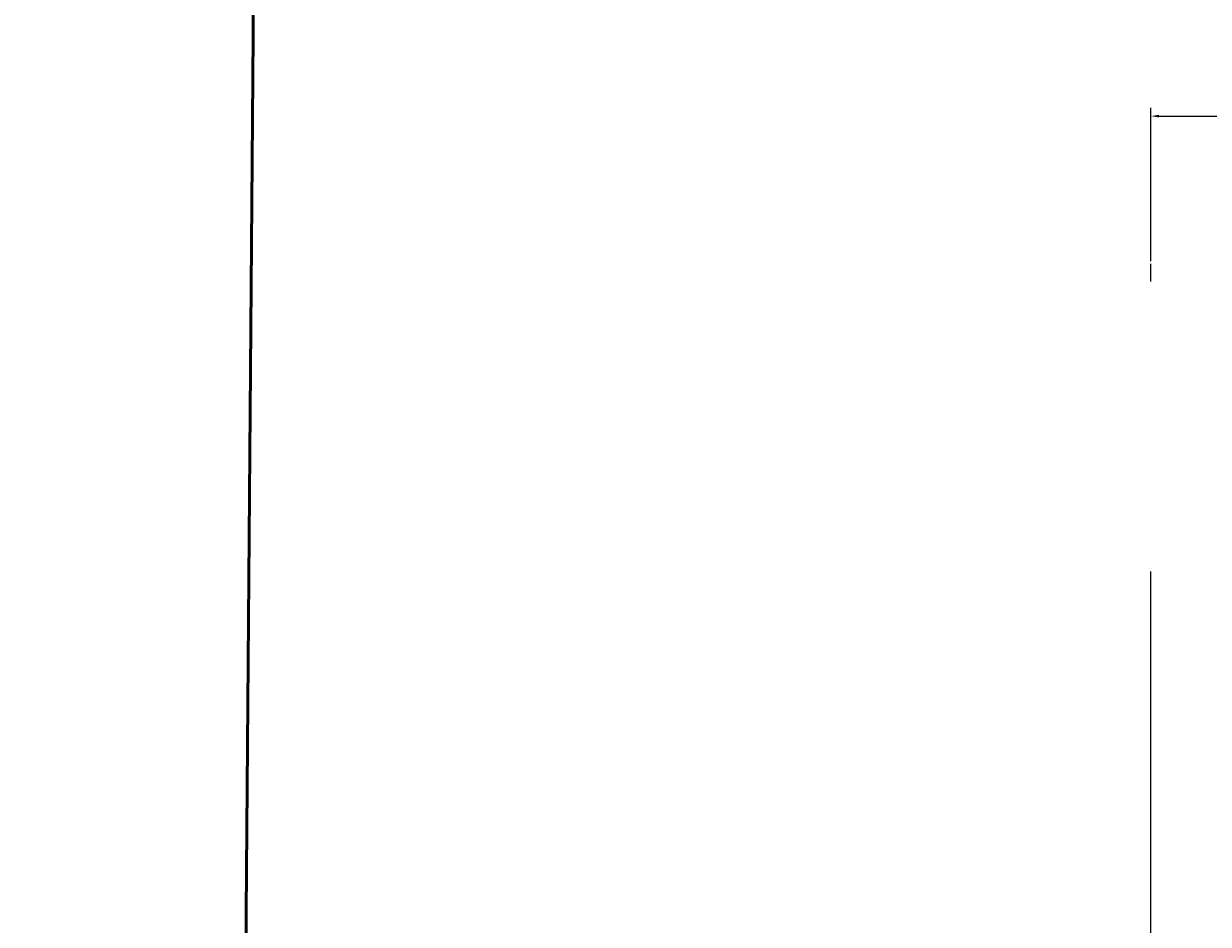
# Model space of a CAD drawing. Units: millimetres. Extents: x -53 to 92, y -147 to 37.
# Tile 11 of 16: x -6 to 20, y -30 to -10. Entities that reach past the tile are written whole.
import ezdxf

# ---------------------------------------------------------------- set-up
doc = ezdxf.new("R2010")
doc.units = ezdxf.units.MM
doc.header["$MEASUREMENT"] = 0
doc.linetypes.add('CENTER', pattern=[50.8, 31.75, -6.35, 6.35, -6.35])
for name, color, linetype, lineweight in [('M-CNTR', 4, 'CENTER', 18), ('M-DIMS', 2, 'Continuous', 25), ('M-OUTL', 7, 'Continuous', 50)]:
    doc.layers.add(name, color=color, linetype=linetype, lineweight=lineweight)
doc.styles.get("Standard").update_dxf_attribs({"font": 'arial.ttf'})
doc.dimstyles.get("Standard").update_dxf_attribs({"dimtxt": 0.18, "dimasz": 0.18, "dimexe": 0.18, "dimexo": 0.0625, "dimgap": 0.09, "dimtad": 0, "dimtih": 1, "dimtoh": 1, "dimdec": 4, "dimzin": 0, "dimdsep": 46, "dimtxsty": 'Standard', "dimcen": 0.09, "dimadec": 0, "dimazin": 0, "dimtfac": 1, "dimtdec": 4, "dimtofl": 0, "dimtmove": 0, "dimatfit": 3, "dimfxl": 1, "dimtolj": 1, "dimtzin": 0, "dimarcsym": 0})

# ---------------------------------------------------------------- blocks, each defined once
blk = doc.blocks.new('*D7')
at = {"layer": 'Defpoints', "color": 0, "transparency": 16777216}
for p in [(9.445, -3.88), (-44.321, -53.98), (18.956, -53.98)]:
    blk.add_point(p, dxfattribs=at)
at = {"layer": 'M-DIMS', "color": 0, "lineweight": -2, "transparency": 16777216}
for p, q in [((9.382, -3.88), (-44.501, -3.88)), ((-44.321, -4.06), (-44.321, -27.308)), ((-44.321, -53.8), (-44.321, -30.552)), ((18.894, -53.98), (-44.501, -53.98))]:
    blk.add_line(p, q, dxfattribs=at)
at = {"layer": 'M-DIMS', "color": 0, "transparency": 16777216}
for points in [[(-44.351, -4.06), (-44.291, -4.06), (-44.321, -3.88)], [(-44.351, -53.8), (-44.291, -53.8), (-44.321, -53.98)]]:
    blk.add_solid(points, dxfattribs=at)
at = {"layer": 'M-DIMS', "color": 0, "transparency": 16777216, "insert": (-44.321, -28.93), "char_height": 0.18, "attachment_point": 5}
blk.add_mtext('\\A1;{\\H16.66667x;50}', dxfattribs=at)
blk = doc.blocks.new('*D10')
at = {"layer": 'Defpoints', "color": 0, "transparency": 16777216}
for p in [(64.593, -18.184), (-26.68, -89.776)]:
    blk.add_point(p, dxfattribs=at)
at = {"layer": 'M-DIMS', "color": 0, "lineweight": -2, "transparency": 16777216}
for p, q in [((77.384, -8.151), (64.734, -18.073)), ((77.564, -8.151), (77.384, -8.151)), ((18.956, -54.07), (18.956, -53.89)), ((18.866, -53.98), (19.046, -53.98))]:
    blk.add_line(p, q, dxfattribs=at)
at = {"layer": 'M-DIMS', "color": 0, "transparency": 16777216}
blk.add_solid([(64.716, -18.05), (64.753, -18.097), (64.593, -18.184)], dxfattribs=at)
at = {"layer": 'M-DIMS', "color": 0, "transparency": 16777216, "insert": (82.599, -8.151), "char_height": 0.18, "attachment_point": 5}
blk.add_mtext('\\A1;{\\H16.66667x;%%C116}', dxfattribs=at)
blk = doc.blocks.new('*D14')
at = {"layer": 'Defpoints', "color": 0, "transparency": 16777216}
for p in [(28.692, -12.346), (18.956, -15.584), (28.692, -16.641)]:
    blk.add_point(p, dxfattribs=at)
at = {"layer": 'M-DIMS', "color": 0, "lineweight": -2, "transparency": 16777216}
for p, q in [((18.956, -15.521), (18.956, -12.166)), ((28.692, -16.578), (28.692, -12.166)), ((19.136, -12.346), (21.732, -12.346)), ((28.512, -12.346), (25.917, -12.346))]:
    blk.add_line(p, q, dxfattribs=at)
at = {"layer": 'M-DIMS', "color": 0, "transparency": 16777216}
for points in [[(19.136, -12.316), (19.136, -12.376), (18.956, -12.346)], [(28.512, -12.316), (28.512, -12.376), (28.692, -12.346)]]:
    blk.add_solid(points, dxfattribs=at)
at = {"layer": 'M-DIMS', "color": 0, "transparency": 16777216, "insert": (23.824, -12.346), "char_height": 0.18, "attachment_point": 5}
blk.add_mtext('\\A1;{\\H16.66667x;10}', dxfattribs=at)
blk = doc.blocks.new('*D17')
at = {"layer": 'Defpoints', "color": 0, "transparency": 16777216}
for p in [(-46.81, 25.909), (28.564, 25.909), (18.165, -111.975)]:
    blk.add_point(p, dxfattribs=at)
at = {"layer": 'M-DIMS', "color": 0, "lineweight": -2, "transparency": 16777216}
for p, q in [((28.502, 25.909), (-46.99, 25.909)), ((-46.81, 25.729), (-46.81, -42.851)), ((-46.81, -111.795), (-46.81, -43.215)), ((18.102, -111.975), (-46.99, -111.975))]:
    blk.add_line(p, q, dxfattribs=at)
at = {"layer": 'M-DIMS', "color": 0, "transparency": 16777216}
for points in [[(-46.84, 25.729), (-46.78, 25.729), (-46.81, 25.909)], [(-46.84, -111.795), (-46.78, -111.795), (-46.81, -111.975)]]:
    blk.add_solid(points, dxfattribs=at)
at = {"layer": 'M-DIMS', "color": 0, "transparency": 16777216, "insert": (-46.81, -43.033), "char_height": 0.18, "attachment_point": 5}
blk.add_mtext('\\A1;137.88', dxfattribs=at)
blk = doc.blocks.new('*D18')
at = {"layer": 'Defpoints', "color": 0, "transparency": 16777216}
for p in [(19.753, 4.014), (18.16, -111.975)]:
    blk.add_point(p, dxfattribs=at)
at = {"layer": 'M-DIMS', "color": 0, "lineweight": -2, "transparency": 16777216}
for p, q in [((18.956, -54.07), (18.956, -53.89)), ((18.866, -53.98), (19.046, -53.98)), ((17.682, -146.771), (18.158, -112.155)), ((17.502, -146.771), (17.682, -146.771))]:
    blk.add_line(p, q, dxfattribs=at)
at = {"layer": 'M-DIMS', "color": 0, "transparency": 16777216}
blk.add_solid([(18.128, -112.154), (18.188, -112.155), (18.16, -111.975)], dxfattribs=at)
at = {"layer": 'M-DIMS', "color": 0, "transparency": 16777216, "insert": (17.115, -146.771), "char_height": 0.18, "attachment_point": 5}
blk.add_mtext('\\A1;∅116', dxfattribs=at)

msp = doc.modelspace()

# ---------------------------------------------------------------- linework, layer by layer
at = {"layer": 'M-CNTR'}
msp.add_line((18.95638, -54.07007), (18.95638, -15.58399), dxfattribs=at)
at = {"layer": 'M-OUTL'}
msp.add_line((-1.07952, -58.41764), (-0.64538, -3.86515), dxfattribs=at)
msp.add_arc((18.95638, -53.98007), 58, 108.3895553, 70.0459142, dxfattribs=at)

# ---------------------------------------------------------------- dimensions: what is measured, and where the dimension line sits
at = {"layer": 'M-DIMS'}
dim = msp.add_linear_dim(base=(-46.8103, 25.90924), p1=(18.16452, -111.97467), p2=(28.56407, 25.90924), angle=90, dimstyle='Standard', override={"dimdec": 2, "dimlfac": 1, "dimrnd": 0, "dimzin": 0, "dimdsep": 46, "dimlunit": 2}, dxfattribs=at)
dim.commit()
dim.dimension.update_dxf_attribs({"geometry": '*D17', "text_midpoint": (-46.8103, -43.03271)})
dim = msp.add_diameter_dim_2p(p1=(19.75275, 4.01446), p2=(18.16001, -111.9746), dimstyle='Standard', override={"dimdec": 0, "dimlfac": 1, "dimrnd": 0, "dimzin": 0, "dimdsep": 46, "dimlunit": 2}, dxfattribs=at)
dim.commit()
dim.dimension.update_dxf_attribs({"geometry": '*D18', "text_midpoint": (17.11548, -146.77132), "dimtype": 163})
dim = msp.add_linear_dim(base=(-44.32095, -53.98007), p1=(9.44461, -3.87977), p2=(18.95638, -53.98007), angle=90, text='{\\H16.66667x;50}', dimstyle='Standard', override={"dimclrd": 0, "dimclre": 0, "dimclrt": 0}, dxfattribs=at)
dim.commit()
dim.dimension.update_dxf_attribs({"geometry": '*D7', "text_midpoint": (-44.32095, -28.92992)})
dim = msp.add_diameter_dim_2p(p1=(-26.67986, -89.77579), p2=(64.59262, -18.18435), text='{\\H16.66667x;%%C116}', dimstyle='Standard', override={"dimclrd": 0, "dimclre": 0, "dimclrt": 0}, dxfattribs=at)
dim.commit()
dim.dimension.update_dxf_attribs({"geometry": '*D10', "text_midpoint": (82.59889, -8.15132), "dimtype": 163})
dim = msp.add_linear_dim(base=(28.69189, -12.34633), p1=(18.95638, -15.58399), p2=(28.69189, -16.64088), text='{\\H16.66667x;10}', dimstyle='Standard', override={"dimclrd": 0, "dimclre": 0, "dimclrt": 0}, dxfattribs=at)
dim.commit()
dim.dimension.update_dxf_attribs({"geometry": '*D14', "text_midpoint": (23.82413, -12.34633)})

doc.saveas('drawing.dxf')
